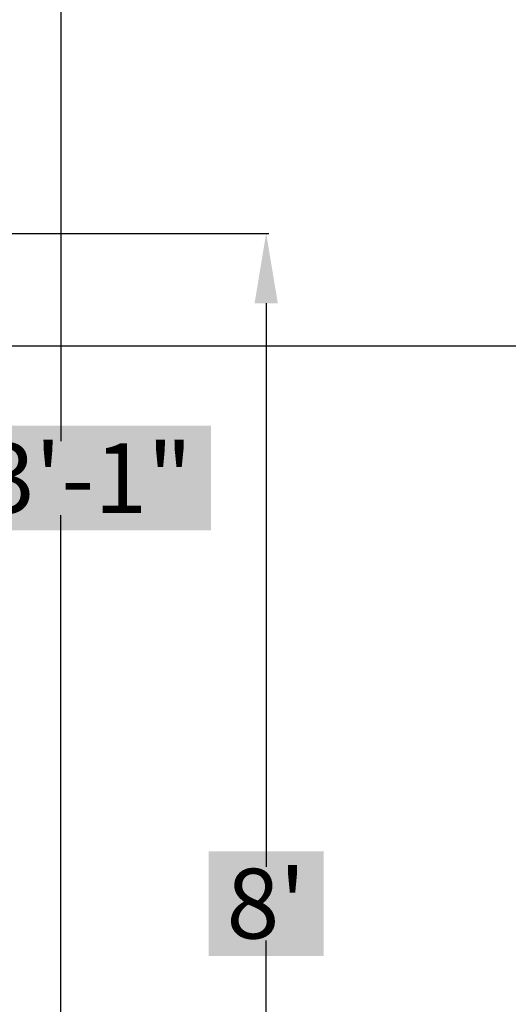
# Model space of a CAD drawing. Units: inches. Extents: x -301 to 715, y -607 to 364.
# Tile 41 of 141: x 159 to 194, y -441 to -370. Entities that reach past the tile are written whole.
import ezdxf

# ---------------------------------------------------------------- set-up
doc = ezdxf.new("R2010")
doc.units = ezdxf.units.IN
doc.header["$MEASUREMENT"] = 0
doc.layers.add('A-ANNO-DIMS', color=2, linetype='Continuous', lineweight=18)
doc.styles.get("Standard").update_dxf_attribs({"font": 'arial.ttf'})
doc.dimstyles.get("Standard").update_dxf_attribs({"dimtxt": 0.18, "dimasz": 0.18, "dimexe": 0.18, "dimexo": 0.0625, "dimgap": 0.09, "dimtad": 0, "dimtih": 1, "dimtoh": 1, "dimdec": 1, "dimzin": 0, "dimdsep": 46, "dimlunit": 4, "dimtxsty": 'Standard', "dimcen": 0.09, "dimclrd": 3, "dimclre": 4, "dimclrt": 6, "dimadec": 0, "dimazin": 0, "dimtfac": 1, "dimtdec": 1, "dimtofl": 0, "dimtmove": 0, "dimatfit": 3, "dimfxl": 1, "dimtfill": 2, "dimtfillclr": 51, "dimtolj": 1, "dimtzin": 0, "dimarcsym": 0})

# ---------------------------------------------------------------- blocks, each defined once
blk = doc.blocks.new('*D76')
at = {"layer": 'A-ANNO-DIMS', "color": 0, "lineweight": -2, "transparency": 16777216}
for p, q in [((158.28, -324.519), (162.311, -324.519)), ((162.131, -329.519), (162.131, -400.354)), ((162.131, -476.477), (162.131, -405.643)), ((158.28, -481.477), (162.311, -481.477))]:
    blk.add_line(p, q, dxfattribs=at)
at = {"layer": 'A-ANNO-DIMS', "color": 0, "transparency": 16777216}
for points in [[(161.297, -329.519), (162.964, -329.519), (162.131, -324.519)], [(161.297, -476.477), (162.964, -476.477), (162.131, -481.477)]]:
    blk.add_solid(points, dxfattribs=at)
at = {"layer": 'Defpoints', "color": 0, "transparency": 16777216}
for p in [(158.218, -324.519), (162.131, -324.519), (158.218, -481.477)]:
    blk.add_point(p, dxfattribs=at)
at = {"layer": 'A-ANNO-DIMS', "color": 0, "transparency": 16777216, "insert": (162.131, -402.998), "char_height": 5, "attachment_point": 5, "bg_fill": 1, "box_fill_scale": 1.25, "bg_fill_color": 51, "bg_fill_transparency": 0}
blk.add_mtext('\\A1;13\'-1"', dxfattribs=at)
blk = doc.blocks.new('*D81')
at = {"layer": 'A-ANNO-DIMS', "color": 0, "lineweight": -2, "transparency": 16777216}
for p, q in [((155.28, -385.477), (177.024, -385.477)), ((176.844, -390.477), (176.844, -430.835)), ((176.844, -476.477), (176.844, -436.12)), ((158.28, -481.477), (177.024, -481.477))]:
    blk.add_line(p, q, dxfattribs=at)
at = {"layer": 'A-ANNO-DIMS', "color": 0, "transparency": 16777216}
for points in [[(176.011, -390.477), (177.678, -390.477), (176.844, -385.477)], [(176.011, -476.477), (177.678, -476.477), (176.844, -481.477)]]:
    blk.add_solid(points, dxfattribs=at)
at = {"layer": 'Defpoints', "color": 0, "transparency": 16777216}
for p in [(155.218, -385.477), (158.218, -481.477), (176.844, -481.477)]:
    blk.add_point(p, dxfattribs=at)
at = {"layer": 'A-ANNO-DIMS', "color": 0, "transparency": 16777216, "insert": (176.844, -433.477), "char_height": 5, "attachment_point": 5, "bg_fill": 1, "box_fill_scale": 1.25, "bg_fill_color": 51, "bg_fill_transparency": 0}
blk.add_mtext("\\A1;8'", dxfattribs=at)
blk = doc.blocks.new('*D176')
at = {"layer": 'A-ANNO-DIMS', "color": 4, "lineweight": -2, "transparency": 16777216}
for p, q in [((148.28, -324.477), (215.605, -324.477)), ((-15.22, -540.477), (215.605, -540.477))]:
    blk.add_line(p, q, dxfattribs=at)
at = {"layer": 'A-ANNO-DIMS', "color": 3, "lineweight": -2, "transparency": 16777216}
for p, q in [((215.425, -324.657), (215.425, -432.296)), ((215.425, -540.297), (215.425, -432.659))]:
    blk.add_line(p, q, dxfattribs=at)
at = {"layer": 'A-ANNO-DIMS', "color": 3, "transparency": 16777216}
for points in [[(215.395, -324.657), (215.455, -324.657), (215.425, -324.477)], [(215.395, -540.297), (215.455, -540.297), (215.425, -540.477)]]:
    blk.add_solid(points, dxfattribs=at)
at = {"layer": 'Defpoints', "color": 0, "transparency": 16777216}
for p in [(148.218, -324.477), (-15.282, -540.477), (215.425, -540.477)]:
    blk.add_point(p, dxfattribs=at)
at = {"layer": 'A-ANNO-DIMS', "color": 6, "transparency": 16777216, "insert": (215.425, -432.477), "char_height": 0.18, "attachment_point": 5, "bg_fill": 1, "box_fill_scale": 1.25, "bg_fill_color": 51, "bg_fill_transparency": 0}
blk.add_mtext('\\A1;18\'-0"', dxfattribs=at)
blk = doc.blocks.new('*D200')
at = {"layer": 'A-ANNO-DIMS', "color": 4, "lineweight": -2, "transparency": 16777216}
for p, q in [((412.955, -393.552), (121.926, -393.552)), ((412.955, -489.552), (121.926, -489.552))]:
    blk.add_line(p, q, dxfattribs=at)
at = {"layer": 'A-ANNO-DIMS', "color": 3, "lineweight": -2, "transparency": 16777216}
for p, q in [((122.106, -393.732), (122.106, -441.371)), ((122.106, -489.372), (122.106, -441.734))]:
    blk.add_line(p, q, dxfattribs=at)
at = {"layer": 'A-ANNO-DIMS', "color": 3, "transparency": 16777216}
for points in [[(122.076, -393.732), (122.136, -393.732), (122.106, -393.552)], [(122.076, -489.372), (122.136, -489.372), (122.106, -489.552)]]:
    blk.add_solid(points, dxfattribs=at)
at = {"layer": 'Defpoints', "color": 0, "transparency": 16777216}
for p in [(122.106, -393.552), (413.018, -393.552), (413.018, -489.552)]:
    blk.add_point(p, dxfattribs=at)
at = {"layer": 'A-ANNO-DIMS', "color": 6, "transparency": 16777216, "insert": (122.106, -441.552), "char_height": 0.18, "attachment_point": 5, "bg_fill": 1, "box_fill_scale": 1.25, "bg_fill_color": 51, "bg_fill_transparency": 0}
blk.add_mtext('\\A1;8\'-0"', dxfattribs=at)

msp = doc.modelspace()

# ---------------------------------------------------------------- dimensions: what is measured, and where the dimension line sits
at = {"layer": 'A-ANNO-DIMS'}
for base, p1, p2, override, picture, middle in [((215.425, -540.477), (148.218, -324.477), (-15.282, -540.477), {"dimdec": 1, "dimlfac": 1, "dimrnd": 0, "dimzin": 1, "dimdsep": 46, "dimlunit": 4, "dimfrac": 2}, '*D176', (215.425, -432.477)), ((162.131, -324.519), (158.218, -481.477), (158.218, -324.519), {"dimtxt": 5, "dimasz": 5, "dimclrd": 0, "dimclre": 0, "dimclrt": 0}, '*D76', (162.131, -402.998)), ((176.844, -481.477), (155.218, -385.477), (158.218, -481.477), {"dimtxt": 5, "dimasz": 5, "dimclrd": 0, "dimclre": 0, "dimclrt": 0}, '*D81', (176.844, -433.477)), ((122.106, -393.552), (413.018, -489.552), (413.018, -393.552), {"dimdec": 1, "dimlfac": 1, "dimrnd": 0, "dimzin": 1, "dimdsep": 46, "dimlunit": 4, "dimfrac": 2}, '*D200', (122.106, -441.552))]:
    dim = msp.add_linear_dim(base=base, p1=p1, p2=p2, angle=90, dimstyle='Standard', override=override, dxfattribs=at)
    dim.commit()
    dim.dimension.update_dxf_attribs({"geometry": picture, "text_midpoint": middle})

doc.saveas('drawing.dxf')
